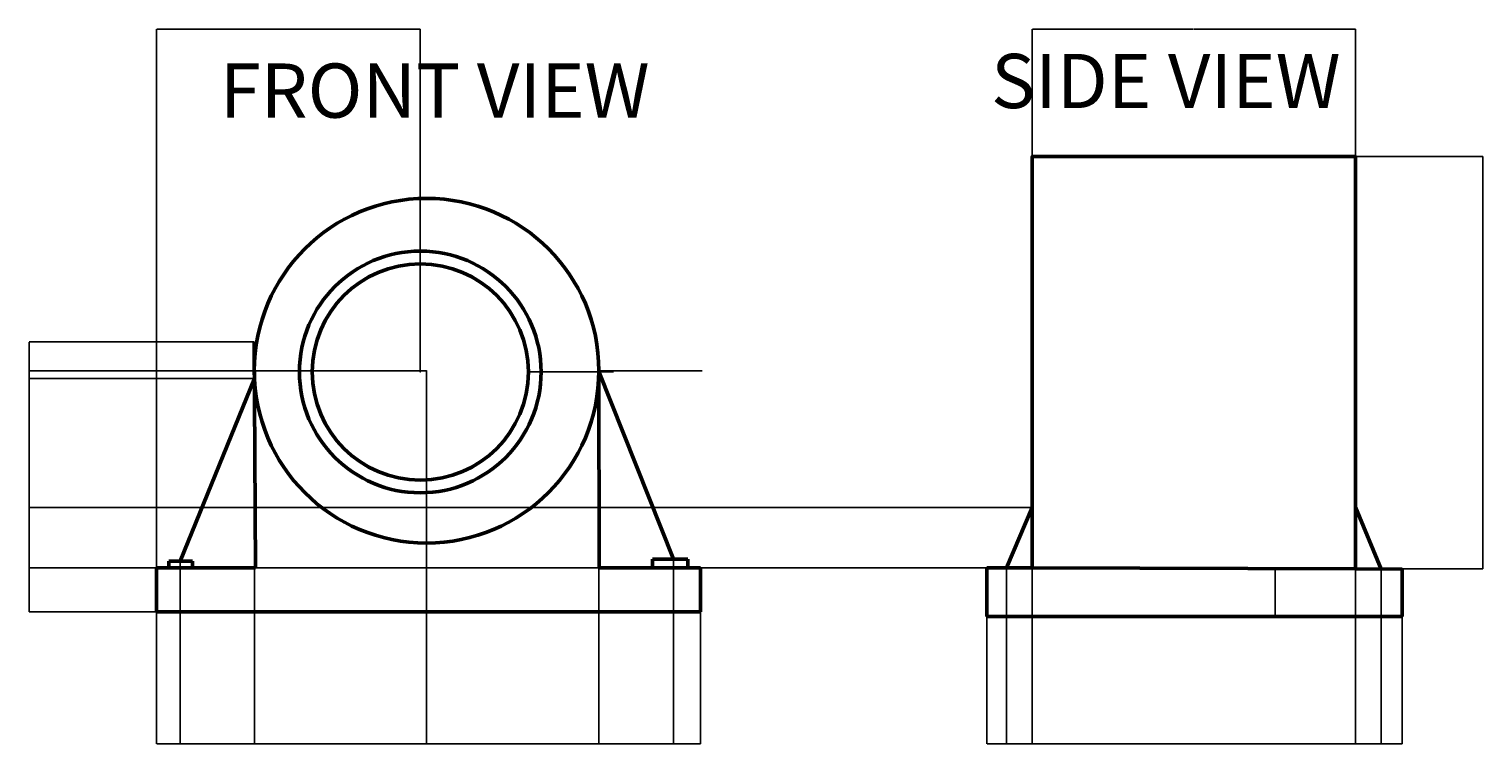
# Model space of a CAD drawing. Units: millimetres. Extents: x 647 to 5260, y 1116 to 2302.
# Tile 1 of 2: x 647 to 3060, y 1116 to 2302. Entities that reach past the tile are written whole.
import ezdxf

# ---------------------------------------------------------------- set-up
doc = ezdxf.new("R2010")
doc.units = ezdxf.units.MM
for name, color, linetype, lineweight in [('M-DIMS', 2, 'Continuous', 18), ('M-OUTL', 7, 'Continuous', 50), ('M-TEXT', 3, 'Continuous', 25)]:
    doc.layers.add(name, color=color, linetype=linetype, lineweight=lineweight)
doc.styles.get("Standard").update_dxf_attribs({"font": 'arial.ttf'})
doc.dimstyles.get("Standard").update_dxf_attribs({"dimtxt": 0.18, "dimasz": 0.18, "dimexe": 0.18, "dimexo": 0.0625, "dimgap": 0.09, "dimtad": 0, "dimtih": 1, "dimtoh": 1, "dimdec": 4, "dimzin": 0, "dimdsep": 46, "dimtxsty": 'Standard', "dimcen": 0.09, "dimadec": 0, "dimazin": 0, "dimtfac": 1, "dimtdec": 4, "dimtofl": 0, "dimtmove": 0, "dimatfit": 3, "dimfxl": 1, "dimtolj": 1, "dimtzin": 0, "dimarcsym": 0})

# ---------------------------------------------------------------- blocks, each defined once
blk = doc.blocks.new('*D1')
at = {"layer": 'Defpoints', "color": 0, "transparency": 16777216}
for p in [(858.7, 1334.7), (1761.8, 1334.7), (1761.8, 1116)]:
    blk.add_point(p, dxfattribs=at)
at = {"layer": 'M-DIMS', "color": 0, "lineweight": -2, "transparency": 16777216}
for p, q in [((858.7, 1334.7), (858.7, 1115.8)), ((1761.8, 1334.7), (1761.8, 1115.8)), ((858.9, 1116), (1309.9, 1116)), ((1761.6, 1116), (1310.6, 1116))]:
    blk.add_line(p, q, dxfattribs=at)
at = {"layer": 'M-DIMS', "color": 0, "transparency": 16777216}
for points in [[(858.9, 1116), (858.9, 1115.9), (858.7, 1116)], [(1761.6, 1116), (1761.6, 1115.9), (1761.8, 1116)]]:
    blk.add_solid(points, dxfattribs=at)
at = {"layer": 'M-DIMS', "color": 0, "transparency": 16777216, "insert": (1310.3, 1116), "char_height": 0.18, "attachment_point": 5}
blk.add_mtext('\\A1;903.1', dxfattribs=at)
blk = doc.blocks.new('*D2')
at = {"layer": 'Defpoints', "color": 0, "transparency": 16777216}
for p in [(647.5, 1735.1), (1306.9, 1735.1), (858.7, 1334.7)]:
    blk.add_point(p, dxfattribs=at)
at = {"layer": 'M-DIMS', "color": 0, "lineweight": -2, "transparency": 16777216}
for p, q in [((1306.9, 1735.1), (647.3, 1735.1)), ((647.5, 1734.9), (647.5, 1535.1)), ((647.5, 1334.9), (647.5, 1534.7)), ((858.7, 1334.7), (647.3, 1334.7))]:
    blk.add_line(p, q, dxfattribs=at)
at = {"layer": 'M-DIMS', "color": 0, "transparency": 16777216}
for points in [[(647.4, 1734.9), (647.5, 1734.9), (647.5, 1735.1)], [(647.4, 1334.9), (647.5, 1334.9), (647.5, 1334.7)]]:
    blk.add_solid(points, dxfattribs=at)
at = {"layer": 'M-DIMS', "color": 0, "transparency": 16777216, "insert": (647.5, 1534.9), "char_height": 0.18, "attachment_point": 5}
blk.add_mtext('\\A1;400.35', dxfattribs=at)
blk = doc.blocks.new('*D3')
at = {"layer": 'Defpoints', "color": 0, "transparency": 16777216}
for p in [(647.5, 1407.8), (858.7, 1407.8), (858.7, 1334.7)]:
    blk.add_point(p, dxfattribs=at)
at = {"layer": 'M-DIMS', "color": 0, "lineweight": -2, "transparency": 16777216}
for p, q in [((858.7, 1407.8), (647.3, 1407.8)), ((647.5, 1407.6), (647.5, 1371.4)), ((647.5, 1334.9), (647.5, 1371.1)), ((858.7, 1334.7), (647.3, 1334.7))]:
    blk.add_line(p, q, dxfattribs=at)
at = {"layer": 'M-DIMS', "color": 0, "transparency": 16777216}
for points in [[(647.4, 1407.6), (647.5, 1407.6), (647.5, 1407.8)], [(647.4, 1334.9), (647.5, 1334.9), (647.5, 1334.7)]]:
    blk.add_solid(points, dxfattribs=at)
at = {"layer": 'M-DIMS', "color": 0, "transparency": 16777216, "insert": (647.5, 1371.3), "char_height": 0.18, "attachment_point": 5}
blk.add_mtext('\\A1;73.02', dxfattribs=at)
blk = doc.blocks.new('*D4')
at = {"layer": 'Defpoints', "color": 0, "transparency": 16777216}
for p in [(1021.2, 1722.4), (858.7, 1407.8), (1021.2, 1116)]:
    blk.add_point(p, dxfattribs=at)
at = {"layer": 'M-DIMS', "color": 0, "lineweight": -2, "transparency": 16777216}
for p, q in [((1021.2, 1722.3), (1021.2, 1115.8)), ((858.7, 1407.7), (858.7, 1115.8)), ((858.9, 1116), (939.6, 1116)), ((1021, 1116), (940.3, 1116))]:
    blk.add_line(p, q, dxfattribs=at)
at = {"layer": 'M-DIMS', "color": 0, "transparency": 16777216}
for points in [[(858.9, 1116), (858.9, 1115.9), (858.7, 1116)], [(1021, 1116), (1021, 1115.9), (1021.2, 1116)]]:
    blk.add_solid(points, dxfattribs=at)
at = {"layer": 'M-DIMS', "color": 0, "transparency": 16777216, "insert": (940, 1116), "char_height": 0.18, "attachment_point": 5}
blk.add_mtext('\\A1;162.5', dxfattribs=at)
blk = doc.blocks.new('*D5')
at = {"layer": 'Defpoints', "color": 0, "transparency": 16777216}
for p in [(1021.2, 1722.4), (1306.9, 1735.1), (1306.9, 1116)]:
    blk.add_point(p, dxfattribs=at)
at = {"layer": 'M-DIMS', "color": 0, "lineweight": -2, "transparency": 16777216}
for p, q in [((1021.2, 1722.3), (1021.2, 1115.8)), ((1306.9, 1735), (1306.9, 1115.8)), ((1021.4, 1116), (1163.6, 1116)), ((1306.8, 1116), (1164.5, 1116))]:
    blk.add_line(p, q, dxfattribs=at)
at = {"layer": 'M-DIMS', "color": 0, "transparency": 16777216}
for points in [[(1021.4, 1116), (1021.4, 1115.9), (1021.2, 1116)], [(1306.8, 1116), (1306.8, 1115.9), (1306.9, 1116)]]:
    blk.add_solid(points, dxfattribs=at)
at = {"layer": 'M-DIMS', "color": 0, "transparency": 16777216, "insert": (1164.1, 1116), "char_height": 0.18, "attachment_point": 5}
blk.add_mtext('\\A1;285.73', dxfattribs=at)
blk = doc.blocks.new('*D6')
at = {"layer": 'Defpoints', "color": 0, "transparency": 16777216}
for p in [(1306.9, 1735.1), (1593, 1733.8), (1593, 1116)]:
    blk.add_point(p, dxfattribs=at)
at = {"layer": 'M-DIMS', "color": 0, "lineweight": -2, "transparency": 16777216}
for p, q in [((1306.9, 1735), (1306.9, 1115.8)), ((1593, 1733.7), (1593, 1115.8)), ((1307.1, 1116), (1449.5, 1116)), ((1592.8, 1116), (1450.4, 1116))]:
    blk.add_line(p, q, dxfattribs=at)
at = {"layer": 'M-DIMS', "color": 0, "transparency": 16777216}
for points in [[(1307.1, 1116), (1307.1, 1115.9), (1306.9, 1116)], [(1592.8, 1116), (1592.8, 1115.9), (1593, 1116)]]:
    blk.add_solid(points, dxfattribs=at)
at = {"layer": 'M-DIMS', "color": 0, "transparency": 16777216, "insert": (1450, 1116), "char_height": 0.18, "attachment_point": 5}
blk.add_mtext('\\A1;286.05', dxfattribs=at)
blk = doc.blocks.new('*D7')
at = {"layer": 'Defpoints', "color": 0, "transparency": 16777216}
for p in [(1593, 1733.8), (1761.8, 1407.8), (1761.8, 1116)]:
    blk.add_point(p, dxfattribs=at)
at = {"layer": 'M-DIMS', "color": 0, "lineweight": -2, "transparency": 16777216}
for p, q in [((1593, 1733.7), (1593, 1115.8)), ((1761.8, 1407.7), (1761.8, 1115.8)), ((1593.2, 1116), (1676.9, 1116)), ((1761.6, 1116), (1677.9, 1116))]:
    blk.add_line(p, q, dxfattribs=at)
at = {"layer": 'M-DIMS', "color": 0, "transparency": 16777216}
for points in [[(1593.2, 1116), (1593.2, 1115.9), (1593, 1116)], [(1761.6, 1116), (1761.6, 1115.9), (1761.8, 1116)]]:
    blk.add_solid(points, dxfattribs=at)
at = {"layer": 'M-DIMS', "color": 0, "transparency": 16777216, "insert": (1677.4, 1116), "char_height": 0.18, "attachment_point": 5}
blk.add_mtext('\\A1;168.84', dxfattribs=at)
blk = doc.blocks.new('*D8')
at = {"layer": 'Defpoints', "color": 0, "transparency": 16777216}
for p in [(1021.2, 1722.4), (898, 1419), (1021.2, 1116)]:
    blk.add_point(p, dxfattribs=at)
at = {"layer": 'M-DIMS', "color": 0, "lineweight": -2, "transparency": 16777216}
for p, q in [((1021.2, 1722.3), (1021.2, 1115.8)), ((898, 1418.9), (898, 1115.8)), ((898.2, 1116), (959.2, 1116)), ((1021, 1116), (960.1, 1116))]:
    blk.add_line(p, q, dxfattribs=at)
at = {"layer": 'M-DIMS', "color": 0, "transparency": 16777216}
for points in [[(898.2, 1116), (898.2, 1115.9), (898, 1116)], [(1021, 1116), (1021, 1115.9), (1021.2, 1116)]]:
    blk.add_solid(points, dxfattribs=at)
at = {"layer": 'M-DIMS', "color": 0, "transparency": 16777216, "insert": (959.6, 1116), "char_height": 0.18, "attachment_point": 5}
blk.add_mtext('\\A1;123.18', dxfattribs=at)
blk = doc.blocks.new('*D9')
at = {"layer": 'Defpoints', "color": 0, "transparency": 16777216}
for p in [(1593, 1733.8), (1716.6, 1422.4), (1716.6, 1116)]:
    blk.add_point(p, dxfattribs=at)
at = {"layer": 'M-DIMS', "color": 0, "lineweight": -2, "transparency": 16777216}
for p, q in [((1593, 1733.7), (1593, 1115.8)), ((1716.6, 1422.4), (1716.6, 1115.8)), ((1593.2, 1116), (1654.4, 1116)), ((1716.4, 1116), (1655.2, 1116))]:
    blk.add_line(p, q, dxfattribs=at)
at = {"layer": 'M-DIMS', "color": 0, "transparency": 16777216}
for points in [[(1593.2, 1116), (1593.2, 1115.9), (1593, 1116)], [(1716.4, 1116), (1716.4, 1115.9), (1716.6, 1116)]]:
    blk.add_solid(points, dxfattribs=at)
at = {"layer": 'M-DIMS', "color": 0, "transparency": 16777216, "insert": (1654.8, 1116), "char_height": 0.18, "attachment_point": 5}
blk.add_mtext('\\A1;123.6', dxfattribs=at)
blk = doc.blocks.new('*D10')
at = {"layer": 'Defpoints', "color": 0, "transparency": 16777216}
for p in [(1296.5, 2301.8), (1296.5, 1733), (858.7, 1407.8)]:
    blk.add_point(p, dxfattribs=at)
at = {"layer": 'M-DIMS', "color": 0, "lineweight": -2, "transparency": 16777216}
for p, q in [((858.7, 1407.8), (858.7, 2302)), ((858.9, 2301.8), (1077.2, 2301.8)), ((1296.4, 2301.8), (1078, 2301.8)), ((1296.5, 1733.1), (1296.5, 2302))]:
    blk.add_line(p, q, dxfattribs=at)
at = {"layer": 'M-DIMS', "color": 0, "transparency": 16777216}
for points in [[(858.9, 2301.9), (858.9, 2301.8), (858.7, 2301.8)], [(1296.4, 2301.9), (1296.4, 2301.8), (1296.5, 2301.8)]]:
    blk.add_solid(points, dxfattribs=at)
at = {"layer": 'M-DIMS', "color": 0, "transparency": 16777216, "insert": (1077.6, 2301.8), "char_height": 0.18, "attachment_point": 5}
blk.add_mtext('\\A1;437.8', dxfattribs=at)
blk = doc.blocks.new('*D11')
at = {"layer": 'Defpoints', "color": 0, "transparency": 16777216}
for p in [(647.5, 1722.4), (1021.2, 1722.4), (858.7, 1334.7)]:
    blk.add_point(p, dxfattribs=at)
at = {"layer": 'M-DIMS', "color": 0, "lineweight": -2, "transparency": 16777216}
for p, q in [((1021.1, 1722.4), (647.3, 1722.4)), ((647.5, 1722.2), (647.5, 1528.7)), ((647.5, 1334.9), (647.5, 1528.4)), ((858.7, 1334.7), (647.3, 1334.7))]:
    blk.add_line(p, q, dxfattribs=at)
at = {"layer": 'M-DIMS', "color": 0, "transparency": 16777216}
for points in [[(647.4, 1722.2), (647.5, 1722.2), (647.5, 1722.4)], [(647.4, 1334.9), (647.5, 1334.9), (647.5, 1334.7)]]:
    blk.add_solid(points, dxfattribs=at)
at = {"layer": 'M-DIMS', "color": 0, "transparency": 16777216, "insert": (647.5, 1528.6), "char_height": 0.18, "attachment_point": 5}
blk.add_mtext('\\A1;387.64', dxfattribs=at)
blk = doc.blocks.new('*D12')
at = {"layer": 'Defpoints', "color": 0, "transparency": 16777216}
for p in [(647.5, 1782.9), (1020.9, 1782.9), (858.7, 1334.7)]:
    blk.add_point(p, dxfattribs=at)
at = {"layer": 'M-DIMS', "color": 0, "lineweight": -2, "transparency": 16777216}
for p, q in [((1020.9, 1782.9), (647.3, 1782.9)), ((647.5, 1782.7), (647.5, 1559)), ((647.5, 1334.9), (647.5, 1558.6)), ((858.7, 1334.7), (647.3, 1334.7))]:
    blk.add_line(p, q, dxfattribs=at)
at = {"layer": 'M-DIMS', "color": 0, "transparency": 16777216}
for points in [[(647.4, 1782.7), (647.5, 1782.7), (647.5, 1782.9)], [(647.4, 1334.9), (647.5, 1334.9), (647.5, 1334.7)]]:
    blk.add_solid(points, dxfattribs=at)
at = {"layer": 'M-DIMS', "color": 0, "transparency": 16777216, "insert": (647.5, 1558.8), "char_height": 0.18, "attachment_point": 5}
blk.add_mtext('\\A1;448.1', dxfattribs=at)
blk = doc.blocks.new('*D13')
at = {"layer": 'Defpoints', "color": 0, "transparency": 16777216}
for p in [(2237.1, 1327.5), (2926.5, 1327.5), (2926.5, 1116)]:
    blk.add_point(p, dxfattribs=at)
at = {"layer": 'M-DIMS', "color": 0, "lineweight": -2, "transparency": 16777216}
for p, q in [((2237.1, 1327.4), (2237.1, 1115.8)), ((2926.5, 1327.4), (2926.5, 1115.8)), ((2237.3, 1116), (2581.4, 1116)), ((2926.3, 1116), (2582.2, 1116))]:
    blk.add_line(p, q, dxfattribs=at)
at = {"layer": 'M-DIMS', "color": 0, "transparency": 16777216}
for points in [[(2237.3, 1116), (2237.3, 1115.9), (2237.1, 1116)], [(2926.3, 1116), (2926.3, 1115.9), (2926.5, 1116)]]:
    blk.add_solid(points, dxfattribs=at)
at = {"layer": 'M-DIMS', "color": 0, "transparency": 16777216, "insert": (2581.8, 1116), "char_height": 0.18, "attachment_point": 5}
blk.add_mtext('\\A1;689.4', dxfattribs=at)
blk = doc.blocks.new('*D14')
at = {"layer": 'Defpoints', "color": 0, "transparency": 16777216}
for p in [(2848.9, 2301.8), (2312.4, 2090.6), (2848.9, 2090.6)]:
    blk.add_point(p, dxfattribs=at)
at = {"layer": 'M-DIMS', "color": 0, "lineweight": -2, "transparency": 16777216}
for p, q in [((2312.4, 2090.6), (2312.4, 2302)), ((2312.6, 2301.8), (2580.2, 2301.8)), ((2848.7, 2301.8), (2581, 2301.8)), ((2848.9, 2090.6), (2848.9, 2302))]:
    blk.add_line(p, q, dxfattribs=at)
at = {"layer": 'M-DIMS', "color": 0, "transparency": 16777216}
for points in [[(2312.6, 2301.9), (2312.6, 2301.8), (2312.4, 2301.8)], [(2848.7, 2301.9), (2848.7, 2301.8), (2848.9, 2301.8)]]:
    blk.add_solid(points, dxfattribs=at)
at = {"layer": 'M-DIMS', "color": 0, "transparency": 16777216, "insert": (2580.6, 2301.8), "char_height": 0.18, "attachment_point": 5}
blk.add_mtext('\\A1;536.5', dxfattribs=at)
blk = doc.blocks.new('*D15')
at = {"layer": 'Defpoints', "color": 0, "transparency": 16777216}
for p in [(2848.9, 2090.6), (2848.9, 1406.1), (3060.1, 1406.1)]:
    blk.add_point(p, dxfattribs=at)
at = {"layer": 'M-DIMS', "color": 0, "lineweight": -2, "transparency": 16777216}
for p, q in [((2848.9, 2090.6), (3060.3, 2090.6)), ((3060.1, 2090.4), (3060.1, 1748.5)), ((3060.1, 1406.3), (3060.1, 1748.1)), ((2848.9, 1406.1), (3060.3, 1406.1))]:
    blk.add_line(p, q, dxfattribs=at)
at = {"layer": 'M-DIMS', "color": 0, "transparency": 16777216}
for points in [[(3060.1, 2090.4), (3060.1, 2090.4), (3060.1, 2090.6)], [(3060.1, 1406.3), (3060.1, 1406.3), (3060.1, 1406.1)]]:
    blk.add_solid(points, dxfattribs=at)
at = {"layer": 'M-DIMS', "color": 0, "transparency": 16777216, "insert": (3060.1, 1748.3), "char_height": 0.18, "attachment_point": 5}
blk.add_mtext('\\A1;684.5', dxfattribs=at)
blk = doc.blocks.new('*D16')
at = {"layer": 'Defpoints', "color": 0, "transparency": 16777216}
for p in [(2715.3, 1405.8), (2926.5, 1405.8), (2926.5, 1327.5)]:
    blk.add_point(p, dxfattribs=at)
at = {"layer": 'M-DIMS', "color": 0, "lineweight": -2, "transparency": 16777216}
for p, q in [((2926.5, 1405.8), (2715.1, 1405.8)), ((2715.3, 1405.7), (2715.3, 1366.8)), ((2715.3, 1327.6), (2715.3, 1366.5)), ((2926.5, 1327.5), (2715.1, 1327.5))]:
    blk.add_line(p, q, dxfattribs=at)
at = {"layer": 'M-DIMS', "color": 0, "transparency": 16777216}
for points in [[(2715.2, 1405.7), (2715.3, 1405.7), (2715.3, 1405.8)], [(2715.2, 1327.6), (2715.3, 1327.6), (2715.3, 1327.5)]]:
    blk.add_solid(points, dxfattribs=at)
at = {"layer": 'M-DIMS', "color": 0, "transparency": 16777216, "insert": (2715.3, 1366.7), "char_height": 0.18, "attachment_point": 5}
blk.add_mtext('\\A1;78.38', dxfattribs=at)
blk = doc.blocks.new('*D17')
at = {"layer": 'Defpoints', "color": 0, "transparency": 16777216}
for p in [(2237.1, 1408), (2269.6, 1407.9), (2269.6, 1116)]:
    blk.add_point(p, dxfattribs=at)
at = {"layer": 'M-DIMS', "color": 0, "lineweight": -2, "transparency": 16777216}
for p, q in [((2237.1, 1407.9), (2237.1, 1115.8)), ((2269.6, 1407.8), (2269.6, 1115.8)), ((2237.3, 1116), (2252.9, 1116)), ((2269.4, 1116), (2253.8, 1116))]:
    blk.add_line(p, q, dxfattribs=at)
at = {"layer": 'M-DIMS', "color": 0, "transparency": 16777216}
for points in [[(2237.3, 1116), (2237.3, 1115.9), (2237.1, 1116)], [(2269.4, 1116), (2269.4, 1115.9), (2269.6, 1116)]]:
    blk.add_solid(points, dxfattribs=at)
at = {"layer": 'M-DIMS', "color": 0, "transparency": 16777216, "insert": (2253.3, 1116), "char_height": 0.18, "attachment_point": 5}
blk.add_mtext('\\A1;32.474', dxfattribs=at)
blk = doc.blocks.new('*D18')
at = {"layer": 'Defpoints', "color": 0, "transparency": 16777216}
for p in [(2269.6, 1407.9), (2312.4, 1407.8), (2312.4, 1116)]:
    blk.add_point(p, dxfattribs=at)
at = {"layer": 'M-DIMS', "color": 0, "lineweight": -2, "transparency": 16777216}
for p, q in [((2269.6, 1407.8), (2269.6, 1115.8)), ((2312.4, 1407.7), (2312.4, 1115.8)), ((2269.8, 1116), (2290.6, 1116)), ((2312.2, 1116), (2291.4, 1116))]:
    blk.add_line(p, q, dxfattribs=at)
at = {"layer": 'M-DIMS', "color": 0, "transparency": 16777216}
for points in [[(2269.8, 1116), (2269.8, 1115.9), (2269.6, 1116)], [(2312.2, 1116), (2312.2, 1115.9), (2312.4, 1116)]]:
    blk.add_solid(points, dxfattribs=at)
at = {"layer": 'M-DIMS', "color": 0, "transparency": 16777216, "insert": (2291, 1116), "char_height": 0.18, "attachment_point": 5}
blk.add_mtext('\\A1;42.82', dxfattribs=at)
blk = doc.blocks.new('*D19')
at = {"layer": 'Defpoints', "color": 0, "transparency": 16777216}
for p in [(2848.9, 1406.1), (2891.3, 1406), (2891.3, 1116)]:
    blk.add_point(p, dxfattribs=at)
at = {"layer": 'M-DIMS', "color": 0, "lineweight": -2, "transparency": 16777216}
for p, q in [((2848.9, 1406), (2848.9, 1115.8)), ((2891.3, 1405.9), (2891.3, 1115.8)), ((2849, 1116), (2869.7, 1116)), ((2891.1, 1116), (2870.5, 1116))]:
    blk.add_line(p, q, dxfattribs=at)
at = {"layer": 'M-DIMS', "color": 0, "transparency": 16777216}
for points in [[(2849, 1116), (2849, 1115.9), (2848.9, 1116)], [(2891.1, 1116), (2891.1, 1115.9), (2891.3, 1116)]]:
    blk.add_solid(points, dxfattribs=at)
at = {"layer": 'M-DIMS', "color": 0, "transparency": 16777216, "insert": (2870.1, 1116), "char_height": 0.18, "attachment_point": 5}
blk.add_mtext('\\A1;42.43', dxfattribs=at)
blk = doc.blocks.new('*D20')
at = {"layer": 'Defpoints', "color": 0, "transparency": 16777216}
for p in [(2891.3, 1406), (2926.5, 1405.8), (2926.5, 1116)]:
    blk.add_point(p, dxfattribs=at)
at = {"layer": 'M-DIMS', "color": 0, "lineweight": -2, "transparency": 16777216}
for p, q in [((2891.3, 1405.9), (2891.3, 1115.8)), ((2926.5, 1405.8), (2926.5, 1115.8)), ((2891.5, 1116), (2908.4, 1116)), ((2926.3, 1116), (2909.4, 1116))]:
    blk.add_line(p, q, dxfattribs=at)
at = {"layer": 'M-DIMS', "color": 0, "transparency": 16777216}
for points in [[(2891.5, 1116), (2891.5, 1115.9), (2891.3, 1116)], [(2926.3, 1116), (2926.3, 1115.9), (2926.5, 1116)]]:
    blk.add_solid(points, dxfattribs=at)
at = {"layer": 'M-DIMS', "color": 0, "transparency": 16777216, "insert": (2908.9, 1116), "char_height": 0.18, "attachment_point": 5}
blk.add_mtext('\\A1;35.224', dxfattribs=at)
blk = doc.blocks.new('*D21')
at = {"layer": 'Defpoints', "color": 0, "transparency": 16777216}
for p in [(647.5, 1508.3), (2312.4, 1508.3), (2269.6, 1407.9)]:
    blk.add_point(p, dxfattribs=at)
at = {"layer": 'M-DIMS', "color": 0, "lineweight": -2, "transparency": 16777216}
for p, q in [((2312.3, 1508.3), (647.3, 1508.3)), ((647.5, 1508.1), (647.5, 1458.3)), ((647.5, 1408.1), (647.5, 1457.9)), ((2269.5, 1407.9), (647.3, 1407.9))]:
    blk.add_line(p, q, dxfattribs=at)
at = {"layer": 'M-DIMS', "color": 0, "transparency": 16777216}
for points in [[(647.4, 1508.1), (647.5, 1508.1), (647.5, 1508.3)], [(647.4, 1408.1), (647.5, 1408.1), (647.5, 1407.9)]]:
    blk.add_solid(points, dxfattribs=at)
at = {"layer": 'M-DIMS', "color": 0, "transparency": 16777216, "insert": (647.5, 1458.1), "char_height": 0.18, "attachment_point": 5}
blk.add_mtext('\\A1;100.4', dxfattribs=at)
blk = doc.blocks.new('*D33')
at = {"layer": 'Defpoints', "color": 0, "transparency": 16777216}
for p in [(1020.9, 1735.1), (1593, 1735.1)]:
    blk.add_point(p, dxfattribs=at)
at = {"layer": 'M-DIMS', "color": 0, "lineweight": -2, "transparency": 16777216}
for p, q in [((1306.8, 1735.1), (1307, 1735.1)), ((1306.9, 1735), (1306.9, 1735.2)), ((1764.6, 1735.1), (1593.1, 1735.1))]:
    blk.add_line(p, q, dxfattribs=at)
at = {"layer": 'M-DIMS', "color": 0, "transparency": 16777216}
blk.add_solid([(1593.1, 1735.1), (1593.1, 1735.1), (1593, 1735.1)], dxfattribs=at)
at = {"layer": 'M-DIMS', "color": 0, "transparency": 16777216, "insert": (1764.9, 1735.1), "char_height": 0.18, "attachment_point": 5}
blk.add_mtext('\\A1;∅572', dxfattribs=at)
blk = doc.blocks.new('*D34')
at = {"layer": 'Defpoints', "color": 0, "transparency": 16777216}
for p in [(1096, 1733), (1497.1, 1733)]:
    blk.add_point(p, dxfattribs=at)
at = {"layer": 'M-DIMS', "color": 0, "lineweight": -2, "transparency": 16777216}
for p, q in [((1296.4, 1733), (1296.6, 1733)), ((1296.5, 1732.9), (1296.5, 1733.1)), ((1617.4, 1733), (1497.3, 1733))]:
    blk.add_line(p, q, dxfattribs=at)
at = {"layer": 'M-DIMS', "color": 0, "transparency": 16777216}
blk.add_solid([(1497.3, 1733), (1497.3, 1733), (1497.1, 1733)], dxfattribs=at)
at = {"layer": 'M-DIMS', "color": 0, "transparency": 16777216, "insert": (1617.9, 1733), "char_height": 0.18, "attachment_point": 5}
blk.add_mtext('\\A1;∅401.1', dxfattribs=at)
blk = doc.blocks.new('*D35')
at = {"layer": 'Defpoints', "color": 0, "transparency": 16777216}
for p in [(1117.2, 1733), (1475.9, 1733)]:
    blk.add_point(p, dxfattribs=at)
at = {"layer": 'M-DIMS', "color": 0, "lineweight": -2, "transparency": 16777216}
for p, q in [((1296.4, 1733), (1296.6, 1733)), ((1296.5, 1732.9), (1296.5, 1733.1)), ((1583.5, 1733), (1476.1, 1733))]:
    blk.add_line(p, q, dxfattribs=at)
at = {"layer": 'M-DIMS', "color": 0, "transparency": 16777216}
blk.add_solid([(1476.1, 1733), (1476.1, 1733), (1475.9, 1733)], dxfattribs=at)
at = {"layer": 'M-DIMS', "color": 0, "transparency": 16777216, "insert": (1584, 1733), "char_height": 0.18, "attachment_point": 5}
blk.add_mtext('\\A1;∅358.7', dxfattribs=at)

msp = doc.modelspace()

# ---------------------------------------------------------------- linework, layer by layer
at = {"layer": 'M-OUTL'}
for p, q in [((1020.9212, 1782.8643), (1022.673, 1407.7591)), ((898.0252, 1419.0096), (1021.2037, 1722.3833)), ((1021.1574, 1732.292), (1020.9349, 1732.2914)), ((1592.9494, 1733.7864), (1592.9842, 1733.7865)), ((1716.5726, 1422.4223), (1592.9494, 1733.7864)), ((1592.9842, 1733.7865), (1593.1947, 1407.7591)), ((2269.5811, 1407.8927), (2312.3986, 1508.2915)), ((2848.8663, 1508.6979), (2891.2975, 1405.9525)), ((917.2606, 1407.7591), (858.7162, 1407.7591)), ((858.7162, 1407.7591), (858.7162, 1334.7428)), ((879.1452, 1407.7591), (879.1401, 1419.0542)), ((879.1401, 1419.0542), (918.5728, 1419.0542)), ((898.0252, 1419.0542), (898.0252, 1419.0096)), ((917.2606, 1407.7591), (1022.673, 1407.7591)), ((918.5728, 1419.0542), (918.5728, 1407.7591)), ((1593.1947, 1407.7591), (1761.8216, 1407.7591)), ((1682.1761, 1407.2058), (1682.1761, 1422.4223)), ((1682.1761, 1422.4223), (1740.855, 1422.4223)), ((1740.855, 1422.4223), (1740.6705, 1407.2058)), ((1761.8216, 1407.7591), (1761.8216, 1334.7428)), ((2237.1073, 1407.9941), (2237.088, 1327.4596)), ((2312.3986, 1407.7591), (2237.1073, 1407.9941)), ((2312.3986, 1407.7591), (2848.8663, 1406.0849)), ((2848.8663, 1406.0849), (2926.522, 1405.8426)), ((2926.522, 1327.4596), (2926.522, 1405.8426)), ((858.7162, 1334.7428), (1761.8216, 1334.7428)), ((2237.088, 1327.4596), (2926.522, 1327.4596))]:
    msp.add_line(p, q, dxfattribs=at)
msp.add_lwpolyline([(2312.3986, 1407.7591), (2312.3986, 2090.5731), (2848.8663, 2090.5731), (2848.8663, 1406.0849)], dxfattribs=at)
for centre, radius in [((1306.9368, 1735.0911), 286.0156), ((1296.5324, 1733.0117), 200.5452), ((1296.5324, 1733.0117), 179.3527)]:
    msp.add_circle(centre, radius, dxfattribs=at)

# ---------------------------------------------------------------- texts
at = {"layer": 'M-TEXT', "char_height": 90, "attachment_point": 1}
for s, insert in [('FRONT VIEW', (963.7589, 2244.9282)), ('SIDE VIEW', (2244.0409, 2260.8799))]:
    msp.add_mtext(s, dxfattribs=dict(at, insert=insert))

# ---------------------------------------------------------------- dimensions: what is measured, and where the dimension line sits
at = {"layer": 'M-DIMS'}
for base, p1, p2, override, picture, middle in [((1296.5324, 2301.8231), (858.7162, 1407.7591), (1296.5324, 1733.0117), {"dimdec": 1, "dimlfac": 1, "dimrnd": 0, "dimzin": 0, "dimdsep": 46, "dimlunit": 2}, '*D10', (1077.6243, 2301.8231)), ((2848.8663, 2301.8231), (2312.3986, 2090.5731), (2848.8663, 2090.5731), {"dimdec": 1, "dimlfac": 1, "dimrnd": 0, "dimzin": 0, "dimdsep": 46, "dimlunit": 2}, '*D14', (2580.6325, 2301.8231)), ((1021.2037, 1115.9773), (858.7162, 1407.7591), (1021.2037, 1722.3833), {"dimdec": 1, "dimlfac": 1, "dimrnd": 0, "dimzin": 0, "dimdsep": 46, "dimlunit": 2}, '*D4', (939.96, 1115.9773)), ((1021.2037, 1115.9773), (898.0252, 1419.0096), (1021.2037, 1722.3833), {"dimdec": 2, "dimlfac": 1, "dimrnd": 0, "dimzin": 0, "dimdsep": 46, "dimlunit": 2}, '*D8', (959.6145, 1115.9773)), ((1306.9368, 1115.9773), (1021.2037, 1722.3833), (1306.9368, 1735.0911), {"dimdec": 2, "dimlfac": 1, "dimrnd": 0, "dimzin": 0, "dimdsep": 46, "dimlunit": 2}, '*D5', (1164.0703, 1115.9773)), ((1592.9842, 1115.9773), (1306.9368, 1735.0911), (1592.9842, 1733.7865), {"dimdec": 2, "dimlfac": 1, "dimrnd": 0, "dimzin": 0, "dimdsep": 46, "dimlunit": 2}, '*D6', (1449.9605, 1115.9773)), ((1761.8216, 1115.9773), (1592.9842, 1733.7865), (1761.8216, 1407.7591), {"dimdec": 2, "dimlfac": 1, "dimrnd": 0, "dimzin": 0, "dimdsep": 46, "dimlunit": 2}, '*D7', (1677.4029, 1115.9773)), ((1716.5726, 1115.9773), (1592.9842, 1733.7865), (1716.5726, 1422.4223), {"dimdec": 1, "dimlfac": 1, "dimrnd": 0, "dimzin": 0, "dimdsep": 46, "dimlunit": 2}, '*D9', (1654.7784, 1115.9773)), ((2269.5811, 1115.9773), (2237.1073, 1407.9941), (2269.5811, 1407.8927), {"dimdec": 3, "dimlfac": 1, "dimrnd": 0, "dimzin": 0, "dimdsep": 46, "dimlunit": 2}, '*D17', (2253.3442, 1115.9773)), ((2312.3986, 1115.9773), (2269.5811, 1407.8927), (2312.3986, 1407.7591), {"dimdec": 2, "dimlfac": 1, "dimrnd": 0, "dimzin": 0, "dimdsep": 46, "dimlunit": 2}, '*D18', (2290.9899, 1115.9773)), ((2891.2975, 1115.9773), (2848.8663, 1406.0849), (2891.2975, 1405.9525), {"dimdec": 2, "dimlfac": 1, "dimrnd": 0, "dimzin": 0, "dimdsep": 46, "dimlunit": 2}, '*D19', (2870.0819, 1115.9773)), ((2926.522037, 1115.977301), (2891.297539, 1405.952533), (2926.522037, 1405.842607), {"dimdec": 3, "dimlfac": 1, "dimrnd": 0, "dimzin": 0, "dimdsep": 46, "dimlunit": 2}, '*D20', (2908.909788, 1115.977301)), ((1761.8216, 1115.9773), (858.7162, 1334.7428), (1761.8216, 1334.7428), {"dimdec": 1, "dimlfac": 1, "dimrnd": 0, "dimzin": 0, "dimdsep": 46, "dimlunit": 2}, '*D1', (1310.2689, 1115.9773)), ((2926.522, 1115.9773), (2237.088, 1327.4596), (2926.522, 1327.4596), {"dimdec": 1, "dimlfac": 1, "dimrnd": 0, "dimzin": 0, "dimdsep": 46, "dimlunit": 2}, '*D13', (2581.805, 1115.9773))]:
    dim = msp.add_linear_dim(base=base, p1=p1, p2=p2, dimstyle='Standard', override=override, dxfattribs=at)
    dim.commit()
    dim.dimension.update_dxf_attribs({"geometry": picture, "text_midpoint": middle})
for base, p1, p2, angle, override, picture, middle in [((3060.1163, 1406.0849), (2848.8663, 2090.5731), (2848.8663, 1406.0849), 270, {"dimdec": 1, "dimlfac": 1, "dimrnd": 0, "dimzin": 0, "dimdsep": 46, "dimlunit": 2}, '*D15', (3060.1163, 1748.329)), ((647.4662, 1782.8643), (858.7162, 1334.7428), (1020.9212, 1782.8643), 90, {"dimdec": 1, "dimlfac": 1, "dimrnd": 0, "dimzin": 0, "dimdsep": 46, "dimlunit": 2}, '*D12', (647.4662, 1558.8035)), ((647.4662, 1735.0911), (858.7162, 1334.7428), (1306.9368, 1735.0911), 90, {"dimdec": 2, "dimlfac": 1, "dimrnd": 0, "dimzin": 0, "dimdsep": 46, "dimlunit": 2}, '*D2', (647.4662, 1534.917)), ((647.4662, 1722.3833), (858.7162, 1334.7428), (1021.2037, 1722.3833), 90, {"dimdec": 2, "dimlfac": 1, "dimrnd": 0, "dimzin": 0, "dimdsep": 46, "dimlunit": 2}, '*D11', (647.4662, 1528.5631)), ((647.4662, 1508.2915), (2269.5811, 1407.8927), (2312.3986, 1508.2915), 90, {"dimdec": 1, "dimlfac": 1, "dimrnd": 0, "dimzin": 0, "dimdsep": 46, "dimlunit": 2}, '*D21', (647.4662, 1458.0921)), ((647.4662, 1407.7591), (858.7162, 1334.7428), (858.7162, 1407.7591), 90, {"dimdec": 2, "dimlfac": 1, "dimrnd": 0, "dimzin": 0, "dimdsep": 46, "dimlunit": 2}, '*D3', (647.4662, 1371.2509)), ((2715.272, 1405.8426), (2926.522, 1327.4596), (2926.522, 1405.8426), 90, {"dimdec": 2, "dimlfac": 1, "dimrnd": 0, "dimzin": 0, "dimdsep": 46, "dimlunit": 2}, '*D16', (2715.272, 1366.6511))]:
    dim = msp.add_linear_dim(base=base, p1=p1, p2=p2, angle=angle, dimstyle='Standard', override=override, dxfattribs=at)
    dim.commit()
    dim.dimension.update_dxf_attribs({"geometry": picture, "text_midpoint": middle})
for p1, p2, override, picture, middle in [((1020.9212, 1735.0913), (1592.9524, 1735.091), {"dimdec": 0, "dimlfac": 1, "dimrnd": 0, "dimzin": 0, "dimdsep": 46, "dimlunit": 2}, '*D33', (1764.5618, 1735.0909)), ((1095.9872, 1733.0114), (1497.0776, 1733.012), {"dimdec": 1, "dimlfac": 1, "dimrnd": 0, "dimzin": 0, "dimdsep": 46, "dimlunit": 2}, '*D34', (1617.4047, 1733.0122)), ((1117.1797, 1733.0114), (1475.8851, 1733.012), {"dimdec": 1, "dimlfac": 1, "dimrnd": 0, "dimzin": 0, "dimdsep": 46, "dimlunit": 2}, '*D35', (1583.4967, 1733.0122))]:
    dim = msp.add_diameter_dim_2p(p1=p1, p2=p2, dimstyle='Standard', override=override, dxfattribs=at)
    dim.commit()
    dim.dimension.update_dxf_attribs({"geometry": picture, "text_midpoint": middle, "dimtype": 163})

doc.saveas('drawing.dxf')
